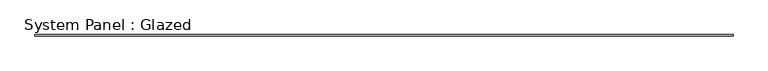
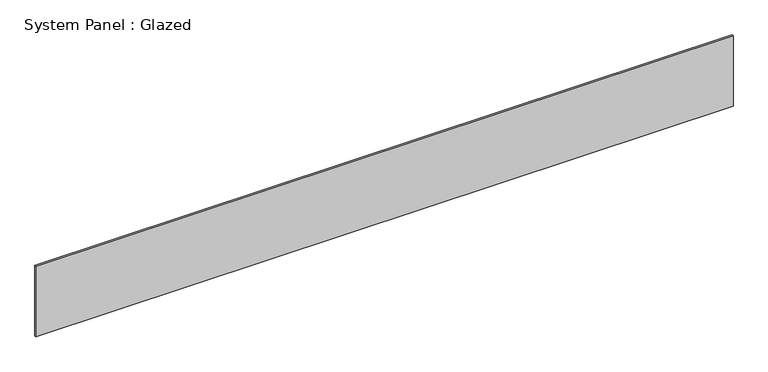
"""IFC4 building model written with IfcOpenShell, lengths in millimetres: plate geometry, System Panel : Glazed."""

from ifc_helpers import new_model, si_unit, origin, origin_with_axes, place, context, project, spatial, polyline, outline, extrude, source, transform, mapped, element, save


def system_panel_glazed_9b7d9a9b(model_context):
    return source(origin(), model_context, "Body", "SweptSolid", [
        extrude(outline(polyline([(6829.6571429, 19.05), (-6829.6571429, 19.05), (-6829.6571429, 44.45), (6829.6571429, 44.45), (6829.6571429, 19.05)])), origin_with_axes(), (0.0, 0.0, 1.0), 1460.5),
    ])


if __name__ == "__main__":
    model = new_model("IFC4")
    model_context = context("Model", 3, world=origin())
    ifc_project = project(units=[si_unit("LENGTHUNIT", "METRE", prefix="MILLI")], contexts=[model_context])
    site = spatial("IfcSite", under=ifc_project)
    building = spatial("IfcBuilding", under=site)
    placement = place(None, origin())
    system_panel_glazed_shape = system_panel_glazed_9b7d9a9b(model_context)
    element("IfcPlate", 1, ObjectType="System Panel : Glazed", at=placement, inside=building, context=model_context, shape_type="MappedRepresentation", body=[
        mapped(system_panel_glazed_shape, transform((0.0, 0.0, 0.0), x_axis=(1.0, 0.0, 0.0), y_axis=(0.0, 1.0, 0.0), z_axis=(0.0, 0.0, 1.0))),
    ])
    save(model, "model.ifc")

# Revit data of these elements
# Type "System Panel : Glazed"
#   Construction Type Id = "GSP4R"
#   Analytic Construction = "1/8 in Pilkington single glazing"
#   Visual Light Transmittance = 0.9
#   Solar Heat Gain Coefficient = 0.86
#   Heat Transfer Coefficient (U) = 1.18115 BTU/(h·ft²·°F)
# Element 1 (IfcPlate, "System Panel : Glazed")
#   Materials on its faces: "Glass"
# Materials
#   "Glass": class "Glass", colour RGB 0 128 192, transparency 0.75, Description = "Soda Lime Glass", Cost = 0
